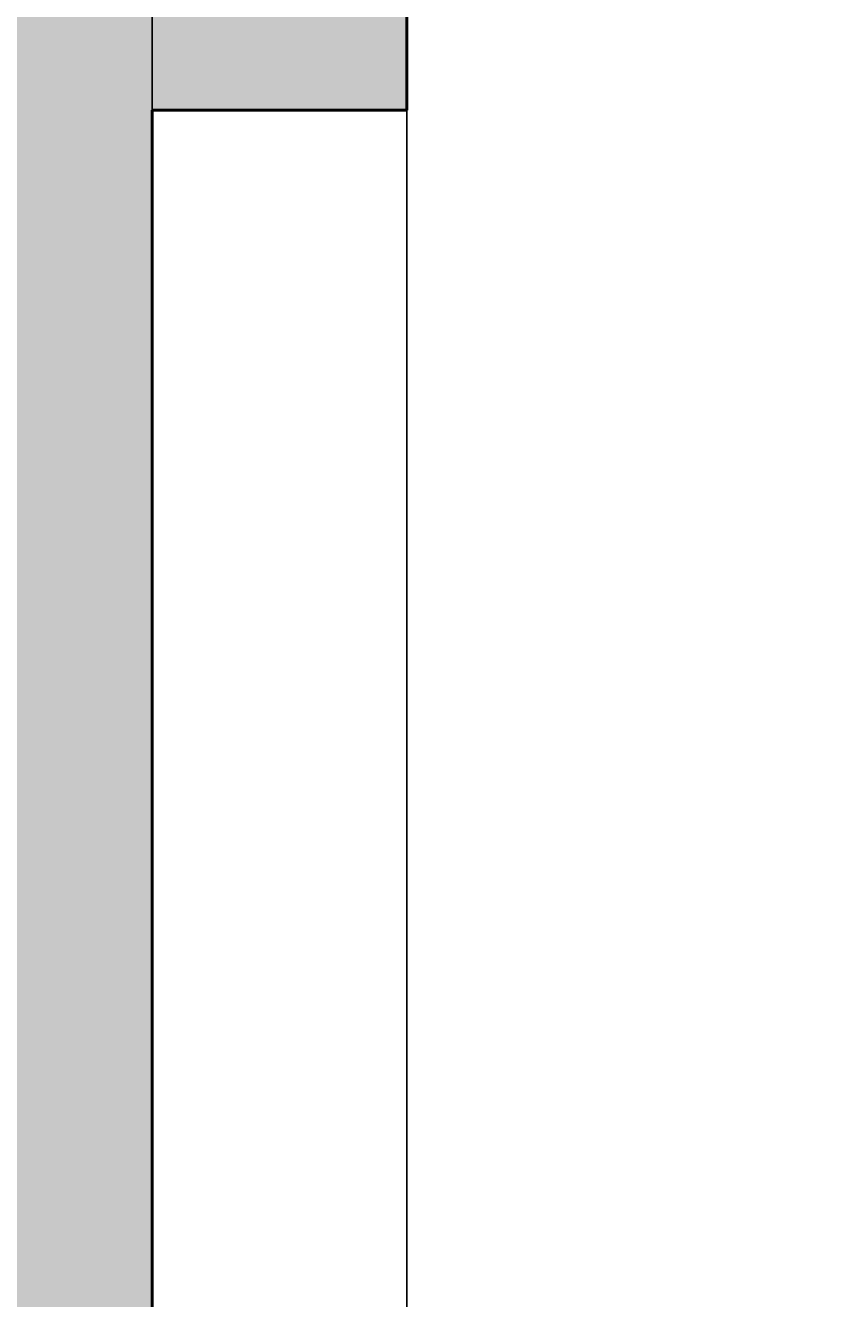
# Model space of a CAD drawing. Units: inches. Extents: x 2307 to 2544, y 2171 to 2540.
# Tile 36 of 52: x 2453 to 2472, y 2407 to 2438. Entities that reach past the tile are written whole.
import ezdxf

# ---------------------------------------------------------------- set-up
doc = ezdxf.new("R2010")
doc.units = ezdxf.units.IN
for name, color, linetype, lineweight in [('A-ANNO-DIMS', 2, 'Continuous', 18), ('A-DOOR', 3, 'Continuous', 25), ('A-WALL', 7, 'Continuous', 50)]:
    doc.layers.add(name, color=color, linetype=linetype, lineweight=lineweight)
doc.layers.add('A-WALL-PATT', color=18, linetype='Continuous', lineweight=13, true_color=0x000000)
doc.styles.get("Standard").update_dxf_attribs({"font": 'arial.ttf'})
doc.dimstyles.get("Standard").update_dxf_attribs({"dimtxt": 0.18, "dimasz": 0.18, "dimexe": 0.18, "dimexo": 0.0625, "dimgap": 0.09, "dimtad": 0, "dimtih": 1, "dimtoh": 1, "dimdec": 4, "dimzin": 0, "dimdsep": 46, "dimtxsty": 'Standard', "dimcen": 0.09, "dimadec": 0, "dimazin": 0, "dimtfac": 1, "dimtdec": 4, "dimtofl": 0, "dimtmove": 0, "dimatfit": 3, "dimfxl": 1, "dimtolj": 1, "dimtzin": 0, "dimarcsym": 0})

# ---------------------------------------------------------------- blocks, each defined once
blk = doc.blocks.new('*U13')
blk.add_line((0, 0), (0, -6))
blk = doc.blocks.new('*D53')
at = {"layer": 'A-ANNO-DIMS', "color": 0, "lineweight": -2, "transparency": 16777216}
for p, q in [((2455.696, 2439.447), (2455.696, 2171.18)), ((2461.696, 2439.447), (2461.696, 2171.18)), ((2455.876, 2171.36), (2458.546, 2171.36)), ((2461.516, 2171.36), (2458.845, 2171.36))]:
    blk.add_line(p, q, dxfattribs=at)
at = {"layer": 'A-ANNO-DIMS', "color": 0, "transparency": 16777216}
for points in [[(2455.876, 2171.39), (2455.876, 2171.33), (2455.696, 2171.36)], [(2461.516, 2171.39), (2461.516, 2171.33), (2461.696, 2171.36)]]:
    blk.add_solid(points, dxfattribs=at)
at = {"layer": 'Defpoints', "color": 0, "transparency": 16777216}
for p in [(2455.696, 2439.51), (2461.696, 2439.51), (2461.696, 2171.36)]:
    blk.add_point(p, dxfattribs=at)
at = {"layer": 'A-ANNO-DIMS', "color": 0, "transparency": 16777216, "insert": (2458.696, 2171.36), "char_height": 0.18, "attachment_point": 5}
blk.add_mtext('\\A1;6', dxfattribs=at)
blk = doc.blocks.new('*D54')
at = {"layer": 'A-ANNO-DIMS', "color": 0, "lineweight": -2, "transparency": 16777216}
for p, q in [((2461.696, 2435.447), (2461.696, 2171.18)), ((2491.696, 2435.447), (2491.696, 2171.18)), ((2461.876, 2171.36), (2476.477, 2171.36)), ((2491.516, 2171.36), (2476.914, 2171.36))]:
    blk.add_line(p, q, dxfattribs=at)
at = {"layer": 'A-ANNO-DIMS', "color": 0, "transparency": 16777216}
for points in [[(2461.876, 2171.39), (2461.876, 2171.33), (2461.696, 2171.36)], [(2491.516, 2171.39), (2491.516, 2171.33), (2491.696, 2171.36)]]:
    blk.add_solid(points, dxfattribs=at)
at = {"layer": 'Defpoints', "color": 0, "transparency": 16777216}
for p in [(2461.696, 2435.51), (2491.696, 2435.51), (2491.696, 2171.36)]:
    blk.add_point(p, dxfattribs=at)
at = {"layer": 'A-ANNO-DIMS', "color": 0, "transparency": 16777216, "insert": (2476.696, 2171.36), "char_height": 0.18, "attachment_point": 5}
blk.add_mtext('\\A1;30', dxfattribs=at)
blk = doc.blocks.new('*D59')
at = {"layer": 'A-ANNO-DIMS', "color": 0, "lineweight": -2, "transparency": 16777216}
for p, q in [((2455.696, 2315.572), (2455.696, 2540.345)), ((2455.876, 2540.165), (2470.477, 2540.165)), ((2485.516, 2540.165), (2470.914, 2540.165)), ((2485.696, 2315.572), (2485.696, 2540.345))]:
    blk.add_line(p, q, dxfattribs=at)
at = {"layer": 'A-ANNO-DIMS', "color": 0, "transparency": 16777216}
for points in [[(2455.876, 2540.195), (2455.876, 2540.135), (2455.696, 2540.165)], [(2485.516, 2540.195), (2485.516, 2540.135), (2485.696, 2540.165)]]:
    blk.add_solid(points, dxfattribs=at)
at = {"layer": 'Defpoints', "color": 0, "transparency": 16777216}
for p in [(2455.696, 2540.165), (2455.696, 2315.51), (2485.696, 2315.51)]:
    blk.add_point(p, dxfattribs=at)
at = {"layer": 'A-ANNO-DIMS', "color": 0, "transparency": 16777216, "insert": (2470.696, 2540.165), "char_height": 0.18, "attachment_point": 5}
blk.add_mtext('\\A1;30', dxfattribs=at)

msp = doc.modelspace()

# ---------------------------------------------------------------- hatches: boundary and pattern name
at = {"layer": 'A-WALL-PATT'}
h = msp.add_hatch(color=256, dxfattribs=at)
h.dxf.hatch_style = 1
h.paths.add_polyline_path([(2433.6935, 2199.5096), (2415.6423, 2199.5096), (2415.6423, 2190.5096), (2433.7832, 2190.5096)], flags=17)
h.paths.add_polyline_path([(2367.6423, 2199.5096), (2335.6958, 2199.5096), (2335.6958, 2307.3983), (2326.6958, 2307.3983), (2326.6958, 2190.5096), (2367.6423, 2190.5096)])
h.paths.add_polyline_path([(2524.6958, 2520.5096), (2496.7832, 2520.5096), (2496.7832, 2515.5149), (2472.7832, 2515.5149), (2472.7832, 2520.5096), (2415.4028, 2520.5096), (2415.4028, 2511.5096), (2451.6958, 2511.5096), (2451.6958, 2439.5096), (2451.6958, 2391.5096), (2445.6958, 2391.5096), (2445.6958, 2387.5096), (2455.6958, 2387.5096), (2455.6958, 2435.5096), (2461.6958, 2435.5096), (2461.6958, 2439.5096), (2455.6958, 2439.5096), (2455.6958, 2511.5096), (2515.6958, 2511.5096), (2515.6958, 2439.5096), (2491.6958, 2439.5096), (2491.6958, 2435.5096), (2515.6958, 2435.5096), (2515.6958, 2319.5096), (2451.6958, 2319.5096), (2451.6958, 2281.5096), (2481.6958, 2281.5096), (2481.6958, 2225.5096), (2485.6958, 2225.5096), (2485.6958, 2285.5096), (2455.6958, 2285.5096), (2455.6958, 2315.5096), (2515.6958, 2315.5096), (2515.6958, 2199.5096), (2469.6952, 2199.5096), (2469.785, 2190.5096), (2524.6958, 2190.5096)])

# ---------------------------------------------------------------- linework, layer by layer
at = {"layer": 'A-WALL'}
for p, q in [((2461.6958, 2439.5096), (2461.6958, 2435.5096)), ((2455.6958, 2387.5096), (2455.6958, 2435.5096)), ((2455.6958, 2435.5096), (2461.6958, 2435.5096)), ((2455.6958, 2435.5096), (2455.6958, 2387.5096))]:
    msp.add_line(p, q, dxfattribs=at)

# ---------------------------------------------------------------- block references
at = {"layer": 'A-DOOR', "xscale": 0.75, "yscale": 0.75, "zscale": 0.75}
msp.add_blockref('*U13', (2461.6958, 2440.0096), dxfattribs=at)

# ---------------------------------------------------------------- dimensions: what is measured, and where the dimension line sits
at = {"layer": 'A-ANNO-DIMS'}
for base, p1, p2, picture, middle in [((2455.6958, 2540.1649), (2485.6958, 2315.5096), (2455.6958, 2315.5096), '*D59', (2470.6958, 2540.1649)), ((2461.6958, 2171.3596), (2455.6958, 2439.5096), (2461.6958, 2439.5096), '*D53', (2458.6958, 2171.3596)), ((2491.6958, 2171.3596), (2461.6958, 2435.5096), (2491.6958, 2435.5096), '*D54', (2476.6958, 2171.3596))]:
    dim = msp.add_linear_dim(base=base, p1=p1, p2=p2, dimstyle='Standard', override={"dimdec": 0, "dimlfac": 1, "dimrnd": 0, "dimzin": 0, "dimdsep": 46, "dimlunit": 2}, dxfattribs=at)
    dim.commit()
    dim.dimension.update_dxf_attribs({"geometry": picture, "text_midpoint": middle})

doc.saveas('drawing.dxf')
